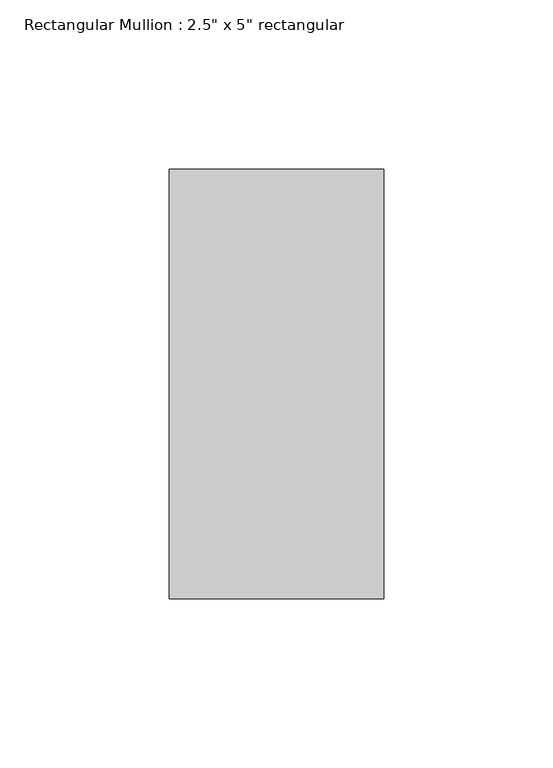
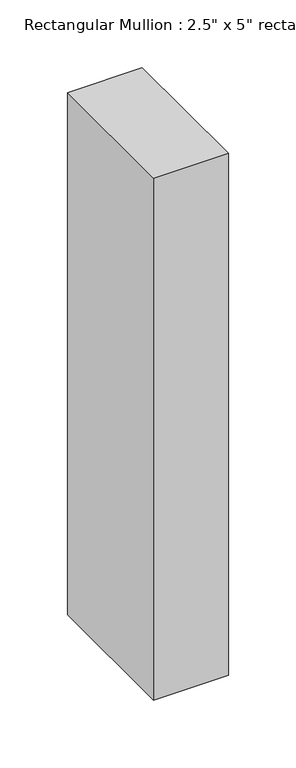
"""IFC4 building model written with IfcOpenShell, lengths in millimetres: member geometry."""

from ifc_helpers import new_model, si_unit, frame, origin, place, context, project, spatial, polyline, outline, extrude, source, transform, mapped, element, save


def member_2b79973d(model_context):
    return source(origin(), model_context, "Body", "SweptSolid", [
        extrude(outline(polyline([(0.0, 63.5), (0.0, -63.5), (-63.5, -63.5), (-63.5, 63.5), (0.0, 63.5)])), frame((0.0, 0.0, -469.9), z_axis=(0.0, 0.0, 1.0), x_axis=(1.0, 0.0, 0.0)), (0.0, 0.0, 1.0), 469.9),
    ])


if __name__ == "__main__":
    model = new_model("IFC4")
    model_context = context("Model", 3, world=origin())
    ifc_project = project(units=[si_unit("LENGTHUNIT", "METRE", prefix="MILLI")], contexts=[model_context])
    site = spatial("IfcSite", under=ifc_project)
    building = spatial("IfcBuilding", under=site)
    placement = place(None, origin())
    member_shape = member_2b79973d(model_context)
    element("IfcMember", 1, ObjectType="Rectangular Mullion : 2.5\" x 5\" rectangular", at=placement, inside=building, context=model_context, shape_type="MappedRepresentation", body=[
        mapped(member_shape, transform((0.0, 0.0, 0.0), x_axis=(1.0, 0.0, 0.0), y_axis=(0.0, 1.0, 0.0), z_axis=(0.0, 0.0, 1.0))),
    ])
    save(model, "model.ifc")

# Revit data of these elements
# Type "Rectangular Mullion : 2.5\" x 5\" rectangular"
#   built-in parameter 1007304 = 0.416667 (stored number, unit not read)
#   built-in parameter 1007301 = 0.104167 (stored number, unit not read)
#   built-in parameter 1007300 = 0.104167 (stored number, unit not read)
# Element 1 (IfcMember, "Rectangular Mullion : 2.5\" x 5\" rectangular")
#   Materials on its faces: "Aluminum"
# Materials
#   "Aluminum": class "Metal", colour RGB 247 247 247, transparency 0, Description = "Aluminum 6061", Cost = 0
